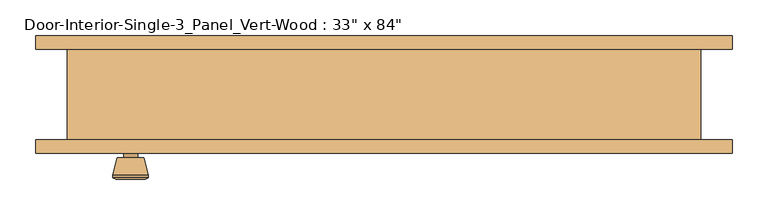
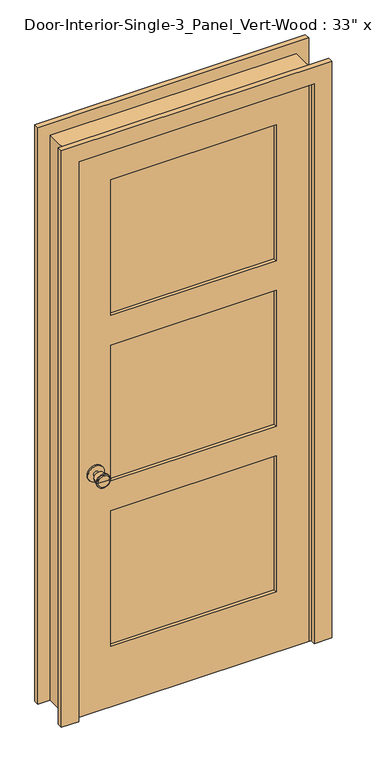
"""IFC4 building model written with IfcOpenShell, lengths in millimetres: door geometry."""

from ifc_helpers import new_model, si_unit, point, frame, frame_2d, origin, place, context, project, spatial, polyline, circle_curve, trimmed, segment, composite_curve, outline, extrude, faceted_brep, source, transform, mapped, element, save
from ifc_brep_helpers import plane_surface, cylinder_surface, revolved_surface, advanced_brep


def door_6500584b(model_context):
    return source(origin(), model_context, "Body", "SolidModel", [
        advanced_brep(
        [(-355.6, -19.4, 914.4), (-365.6, -19.4, 914.4), (-345.6, -19.4, 914.4), (-335.1241324, 29.6, 914.4), (-376.0758676, 29.6, 914.4), (-355.6, 29.6, 914.4), (-330.6, 27.7721319, 914.4), (-380.6, 27.7721319, 914.4), (-330.6, 24.3084537, 914.4), (-380.6, 24.3084537, 914.4), (-336.963764, -0.4, 914.4), (-374.236236, -0.4, 914.4), (-345.6, -0.4, 914.4), (-365.6, -0.4, 914.4)],
        [
            (0, 1),
            (1, 2, circle_curve(frame((-355.6, -19.4, 914.4), z_axis=(0.0, -1.0, 0.0), x_axis=(-1.0, 0.0, 0.0)), 10.0)),
            (2, 0),
            (2, 1, circle_curve(frame((-355.6, -19.4, 914.4), z_axis=(0.0, -1.0, 0.0), x_axis=(-1.0, 0.0, 0.0)), 10.0)),
            (3, 4, circle_curve(frame((-355.6, 29.6, 914.4), z_axis=(0.0, 1.0, 0.0), x_axis=(-1.0, 0.0, 0.0)), 20.4758676)),
            (4, 5),
            (5, 3),
            (4, 3, circle_curve(frame((-355.6, 29.6, 914.4), z_axis=(0.0, 1.0, 0.0), x_axis=(-1.0, 0.0, 0.0)), 20.4758676)),
            (6, 7, circle_curve(frame((-355.6, 27.7721319, 914.4), z_axis=(0.0, 1.0, 0.0), x_axis=(-1.0, 0.0, 0.0)), 25.0)),
            (7, 4),
            (3, 6),
            (7, 6, circle_curve(frame((-355.6, 27.7721319, 914.4), z_axis=(0.0, 1.0, 0.0), x_axis=(-1.0, 0.0, 0.0)), 25.0)),
            (8, 9, circle_curve(frame((-355.6, 24.3084537, 914.4), z_axis=(0.0, 1.0, 0.0), x_axis=(-1.0, 0.0, 0.0)), 25.0)),
            (9, 7),
            (6, 8),
            (9, 8, circle_curve(frame((-355.6, 24.3084537, 914.4), z_axis=(0.0, 1.0, 0.0), x_axis=(-1.0, 0.0, 0.0)), 25.0)),
            (10, 11, circle_curve(frame((-355.6, -0.4, 914.4), z_axis=(0.0, 1.0, 0.0), x_axis=(-1.0, 0.0, 0.0)), 18.636236)),
            (11, 9),
            (8, 10),
            (11, 10, circle_curve(frame((-355.6, -0.4, 914.4), z_axis=(0.0, 1.0, 0.0), x_axis=(-1.0, 0.0, 0.0)), 18.636236)),
            (12, 13, circle_curve(frame((-355.6, -0.4, 914.4), z_axis=(0.0, 1.0, 0.0), x_axis=(-1.0, 0.0, 0.0)), 10.0)),
            (13, 11),
            (10, 12),
            (13, 12, circle_curve(frame((-355.6, -0.4, 914.4), z_axis=(0.0, 1.0, 0.0), x_axis=(-1.0, 0.0, 0.0)), 10.0)),
            (1, 13),
            (12, 2),
        ],
        [
            plane_surface(frame((-355.6, -19.4, 914.4), z_axis=(0.0, -1.0, 0.0), x_axis=(-1.0, 0.0, 0.0))),
            plane_surface(frame((-355.6, 29.6, 914.4), z_axis=(0.0, 1.0, 0.0), x_axis=(-1.0, 0.0, 0.0))),
            revolved_surface(polyline([(-376.0758676, 29.6, 914.4), (-380.6, 27.7721319, 914.4)]), (-355.6, -19.4, 914.4), (0.0, -1.0, 0.0)),
            cylinder_surface(frame((-355.6, -19.4, 914.4), z_axis=(0.0, -1.0, 0.0), x_axis=(-1.0, 0.0, 0.0)), 25.0),
            revolved_surface(polyline([(-380.6, 24.3084537, 914.4), (-374.236236, -0.4, 914.4)]), (-355.6, -19.4, 914.4), (0.0, -1.0, 0.0)),
            plane_surface(frame((-355.6, -0.4, 914.4), z_axis=(0.0, -1.0, 0.0), x_axis=(-1.0, 0.0, 0.0))),
            cylinder_surface(frame((-355.6, -19.4, 914.4), z_axis=(0.0, -1.0, 0.0), x_axis=(-1.0, 0.0, 0.0)), 10.0),
        ],
        [
            (0, [[1, 2, 3]]),
            (0, [[-3, 4, -1]]),
            (1, [[5, 6, 7]]),
            (1, [[8, -7, -6]]),
            (2, [[9, 10, -5, 11]]),
            (2, [[12, -11, -8, -10]]),
            (3, [[13, 14, -9, 15]]),
            (3, [[16, -15, -12, -14]]),
            (4, [[17, 18, -13, 19]]),
            (4, [[20, -19, -16, -18]]),
            (5, [[21, 22, -17, 23]]),
            (5, [[24, -23, -20, -22]]),
            (6, [[-2, 25, -21, 26]]),
            (6, [[-4, -26, -24, -25]]),
        ],
    ),
        extrude(outline(composite_curve([segment(trimmed(circle_curve(frame_2d((914.4, -355.6)), 30.0), [point((914.4, -385.6))], [point((914.4, -325.6))], False, "CARTESIAN"), True, "CONTINUOUS"), segment(trimmed(circle_curve(frame_2d((914.4, -355.6)), 30.0), [point((914.4, -325.6))], [point((914.4, -385.6))], False, "CARTESIAN"), True, "CONTINUOUS")], self_intersect=False)), frame((0.0, -25.4, 0.0), z_axis=(0.0, 1.0, 0.0), x_axis=(0.0, 0.0, 1.0)), (0.0, 0.0, 1.0), 6.0),
        advanced_brep(
        [(-355.6, -66.325, 914.4), (-345.6, -66.325, 914.4), (-365.6, -66.325, 914.4), (-335.1241324, -115.325, 914.4), (-355.6, -115.325, 914.4), (-376.0758676, -115.325, 914.4), (-330.6, -113.4971319, 914.4), (-380.6, -113.4971319, 914.4), (-330.6, -110.0334537, 914.4), (-380.6, -110.0334537, 914.4), (-336.963764, -85.325, 914.4), (-374.236236, -85.325, 914.4), (-345.6, -85.325, 914.4), (-365.6, -85.325, 914.4)],
        [
            (0, 1),
            (1, 2, circle_curve(frame((-355.6, -66.325, 914.4), z_axis=(0.0, 1.0, 0.0), x_axis=(-1.0, 0.0, 0.0)), 10.0)),
            (2, 0),
            (2, 1, circle_curve(frame((-355.6, -66.325, 914.4), z_axis=(0.0, 1.0, 0.0), x_axis=(-1.0, 0.0, 0.0)), 10.0)),
            (3, 4),
            (4, 5),
            (5, 3, circle_curve(frame((-355.6, -115.325, 914.4), z_axis=(0.0, -1.0, 0.0), x_axis=(-1.0, 0.0, 0.0)), 20.4758676)),
            (3, 5, circle_curve(frame((-355.6, -115.325, 914.4), z_axis=(0.0, -1.0, 0.0), x_axis=(-1.0, 0.0, 0.0)), 20.4758676)),
            (6, 3),
            (5, 7),
            (7, 6, circle_curve(frame((-355.6, -113.4971319, 914.4), z_axis=(0.0, -1.0, 0.0), x_axis=(-1.0, 0.0, 0.0)), 25.0)),
            (6, 7, circle_curve(frame((-355.6, -113.4971319, 914.4), z_axis=(0.0, -1.0, 0.0), x_axis=(-1.0, 0.0, 0.0)), 25.0)),
            (8, 6),
            (7, 9),
            (9, 8, circle_curve(frame((-355.6, -110.0334537, 914.4), z_axis=(0.0, -1.0, 0.0), x_axis=(-1.0, 0.0, 0.0)), 25.0)),
            (8, 9, circle_curve(frame((-355.6, -110.0334537, 914.4), z_axis=(0.0, -1.0, 0.0), x_axis=(-1.0, 0.0, 0.0)), 25.0)),
            (10, 8),
            (9, 11),
            (11, 10, circle_curve(frame((-355.6, -85.325, 914.4), z_axis=(0.0, -1.0, 0.0), x_axis=(-1.0, 0.0, 0.0)), 18.636236)),
            (10, 11, circle_curve(frame((-355.6, -85.325, 914.4), z_axis=(0.0, -1.0, 0.0), x_axis=(-1.0, 0.0, 0.0)), 18.636236)),
            (12, 10),
            (11, 13),
            (13, 12, circle_curve(frame((-355.6, -85.325, 914.4), z_axis=(0.0, -1.0, 0.0), x_axis=(-1.0, 0.0, 0.0)), 10.0)),
            (12, 13, circle_curve(frame((-355.6, -85.325, 914.4), z_axis=(0.0, -1.0, 0.0), x_axis=(-1.0, 0.0, 0.0)), 10.0)),
            (1, 12),
            (13, 2),
        ],
        [
            plane_surface(frame((-355.6, -66.325, 914.4), z_axis=(0.0, 1.0, 0.0), x_axis=(-1.0, 0.0, 0.0))),
            plane_surface(frame((-355.6, -115.325, 914.4), z_axis=(0.0, -1.0, 0.0), x_axis=(-1.0, 0.0, 0.0))),
            revolved_surface(polyline([(-376.0758676, -115.325, 914.4), (-380.6, -113.4971319, 914.4)]), (-355.6, -66.325, 914.4), (0.0, 1.0, 0.0)),
            cylinder_surface(frame((-355.6, -66.325, 914.4), z_axis=(0.0, 1.0, 0.0), x_axis=(-1.0, 0.0, 0.0)), 25.0),
            revolved_surface(polyline([(-380.6, -110.0334537, 914.4), (-374.236236, -85.325, 914.4)]), (-355.6, -66.325, 914.4), (0.0, 1.0, 0.0)),
            plane_surface(frame((-355.6, -85.325, 914.4), z_axis=(0.0, 1.0, 0.0), x_axis=(-1.0, 0.0, 0.0))),
            cylinder_surface(frame((-355.6, -66.325, 914.4), z_axis=(0.0, 1.0, 0.0), x_axis=(-1.0, 0.0, 0.0)), 10.0),
        ],
        [
            (0, [[1, 2, 3]]),
            (0, [[-3, 4, -1]]),
            (1, [[5, 6, 7]]),
            (1, [[-6, -5, 8]]),
            (2, [[9, -7, 10, 11]]),
            (2, [[-10, -8, -9, 12]]),
            (3, [[13, -11, 14, 15]]),
            (3, [[-14, -12, -13, 16]]),
            (4, [[17, -15, 18, 19]]),
            (4, [[-18, -16, -17, 20]]),
            (5, [[21, -19, 22, 23]]),
            (5, [[-22, -20, -21, 24]]),
            (6, [[25, -23, 26, -2]]),
            (6, [[-26, -24, -25, -4]]),
        ],
    ),
        extrude(outline(composite_curve([segment(trimmed(circle_curve(frame_2d((914.4, -355.6)), 30.0), [point((914.4, -385.6))], [point((914.4, -325.6))], False, "CARTESIAN"), True, "CONTINUOUS"), segment(trimmed(circle_curve(frame_2d((914.4, -355.6)), 30.0), [point((914.4, -325.6))], [point((914.4, -385.6))], False, "CARTESIAN"), True, "CONTINUOUS")], self_intersect=False)), frame((0.0, -66.325, 0.0), z_axis=(0.0, 1.0, 0.0), x_axis=(0.0, 0.0, 1.0)), (0.0, 0.0, 1.0), 6.0),
        faceted_brep([(444.5, -60.325, 0.0), (419.1, -60.325, 0.0), (419.1, -25.4, 0.0), (406.4, -25.4, 0.0), (406.4, 9.525, 0.0), (419.1, 9.525, 0.0), (419.1, 66.675, 0.0), (444.5, 66.675, 0.0), (444.5, 66.675, 2159.0), (444.5, -60.325, 2159.0), (419.1, 66.675, 2133.6), (-419.1, 66.675, 2133.6), (-419.1, 66.675, 0.0), (-444.5, 66.675, 0.0), (-444.5, 66.675, 2159.0), (419.1, 9.525, 2133.6), (406.4, 9.525, 2120.9), (-406.4, 9.525, 2120.9), (-406.4, 9.525, 0.0), (-419.1, 9.525, 0.0), (-419.1, 9.525, 2133.6), (406.4, -25.4, 2120.9), (419.1, -25.4, 2133.6), (-419.1, -25.4, 2133.6), (-419.1, -25.4, 0.0), (-406.4, -25.4, 0.0), (-406.4, -25.4, 2120.9), (419.1, -60.325, 2133.6), (-444.5, -60.325, 2159.0), (-444.5, -60.325, 0.0), (-419.1, -60.325, 0.0), (-419.1, -60.325, 2133.6)], [[[0, 1, 2, 3, 4, 5, 6, 7]], [[7, 8, 9, 0]], [[6, 10, 11, 12, 13, 14, 8, 7]], [[5, 15, 10, 6]], [[4, 16, 17, 18, 19, 20, 15, 5]], [[3, 21, 16, 4]], [[2, 22, 23, 24, 25, 26, 21, 3]], [[1, 27, 22, 2]], [[0, 9, 28, 29, 30, 31, 27, 1]], [[8, 14, 28, 9]], [[15, 20, 11, 10]], [[21, 26, 17, 16]], [[27, 31, 23, 22]], [[29, 13, 12, 19, 18, 25, 24, 30]], [[14, 13, 29, 28]], [[20, 19, 12, 11]], [[26, 25, 18, 17]], [[31, 30, 24, 23]]]),
        extrude(outline(polyline([(2133.6, -419.1), (0.0, -419.1), (0.0, 419.1), (2133.6, 419.1), (2133.6, -419.1)]), holes=[polyline([(2014.5375, -298.45), (2014.5375, 298.45), (1496.4833333, 298.45), (1496.4833333, -298.45), (2014.5375, -298.45)]), polyline([(749.8291667, -298.45), (749.8291667, 298.45), (231.775, 298.45), (231.775, -298.45), (749.8291667, -298.45)]), polyline([(1382.1833333, -298.45), (1382.1833333, 298.45), (864.1291667, 298.45), (864.1291667, -298.45), (1382.1833333, -298.45)])]), frame((0.0, -60.325, 0.0), z_axis=(0.0, 1.0, 0.0), x_axis=(0.0, 0.0, 1.0)), (0.0, 0.0, 1.0), 34.925),
        extrude(outline(polyline([(298.45, -37.0416667), (298.45, -48.6833333), (-298.45, -48.6833333), (-298.45, -37.0416667), (298.45, -37.0416667)])), frame((0.0, 0.0, 1496.4833333), z_axis=(0.0, 0.0, 1.0), x_axis=(1.0, 0.0, 0.0)), (0.0, 0.0, 1.0), 518.0541667),
        extrude(outline(polyline([(298.45, -37.0416667), (298.45, -48.6833333), (-298.45, -48.6833333), (-298.45, -37.0416667), (298.45, -37.0416667)])), frame((0.0, 0.0, 231.775), z_axis=(0.0, 0.0, 1.0), x_axis=(1.0, 0.0, 0.0)), (0.0, 0.0, 1.0), 518.0541667),
        extrude(outline(polyline([(298.45, -37.0416667), (298.45, -48.6833333), (-298.45, -48.6833333), (-298.45, -37.0416667), (298.45, -37.0416667)])), frame((0.0, 0.0, 864.1291667), z_axis=(0.0, 0.0, 1.0), x_axis=(1.0, 0.0, 0.0)), (0.0, 0.0, 1.0), 518.0541667),
        extrude(outline(polyline([(0.0, 488.95), (2203.45, 488.95), (2203.45, -488.95), (0.0, -488.95), (0.0, -425.45), (2139.95, -425.45), (2139.95, 425.45), (0.0, 425.45), (0.0, 488.95)])), frame((0.0, -79.375, 0.0), z_axis=(0.0, 1.0, 0.0), x_axis=(0.0, 0.0, 1.0)), (0.0, 0.0, 1.0), 19.05),
        extrude(outline(polyline([(0.0, 488.95), (2203.45, 488.95), (2203.45, -488.95), (0.0, -488.95), (0.0, -425.45), (2139.95, -425.45), (2139.95, 425.45), (0.0, 425.45), (0.0, 488.95)])), frame((0.0, 66.675, 0.0), z_axis=(0.0, 1.0, 0.0), x_axis=(0.0, 0.0, 1.0)), (0.0, 0.0, 1.0), 19.05),
    ])


if __name__ == "__main__":
    model = new_model("IFC4")
    model_context = context("Model", 3, world=origin())
    ifc_project = project(units=[si_unit("LENGTHUNIT", "METRE", prefix="MILLI")], contexts=[model_context])
    site = spatial("IfcSite", under=ifc_project)
    building = spatial("IfcBuilding", under=site)
    placement = place(None, origin())
    door_shape = door_6500584b(model_context)
    element("IfcDoor", 1, ObjectType="Door-Interior-Single-3_Panel_Vert-Wood : 33\" x 84\"", at=placement, inside=building, context=model_context, shape_type="MappedRepresentation", body=[
        mapped(door_shape, transform((0.0, 0.0, 0.0), x_axis=(1.0, 0.0, 0.0), y_axis=(0.0, 1.0, 0.0), z_axis=(0.0, 0.0, 1.0))),
    ])
    save(model, "model.ifc")

# Revit data of these elements
# Type "Door-Interior-Single-3_Panel_Vert-Wood : 33\" x 84\""
#   Type Mark = "11"
#   Assembly Code = "C1020300"
#   Analytic Construction = "Wooden"
#   Top Rail = 0' - 4 11/16"
#   Thickness = 0' - 1 3/8"
#   Thermal Resistance (R) = 2.5876 (h·ft²·°F)/BTU
#   Swing Angle [instance default] = 90.00°
#   Stiles = 0' - 4 3/4"
#   Rough Width = 2' - 11"
#   Rough Height = 7' - 1"
#   Intermediate Rail = 0' - 4 1/2"
#   Height = 7' - 0"
#   Width = 2' - 9"
#   Heat Transfer Coefficient (U) = 0.3865 BTU/(h·ft²·°F)
#   Bottom Rail = 0' - 9 1/8"
#   Trim Material = Cherry
#   Panel Material = Cherry
#   Frame Material = Cherry
#   Door Handle Material = Aluminum
#   Visual Light Transmittance = 0
#   Solar Heat Gain Coefficient = 0
#   Wall Closure = (empty or 0)
#   Function = (empty or 0)
# Element 1 (IfcDoor, "Door-Interior-Single-3_Panel_Vert-Wood : 33\" x 84\"")
#   Materials on its faces: "Cherry", "Aluminum"
# Materials
#   "Cherry": class "Wood", colour RGB 226 177 128, transparency 0, Description = "Prunus Serotina", Cost = 0
#   "Aluminum": class "Metal", colour RGB 247 247 247, transparency 0, Description = "Aluminum 6061", Cost = 0
